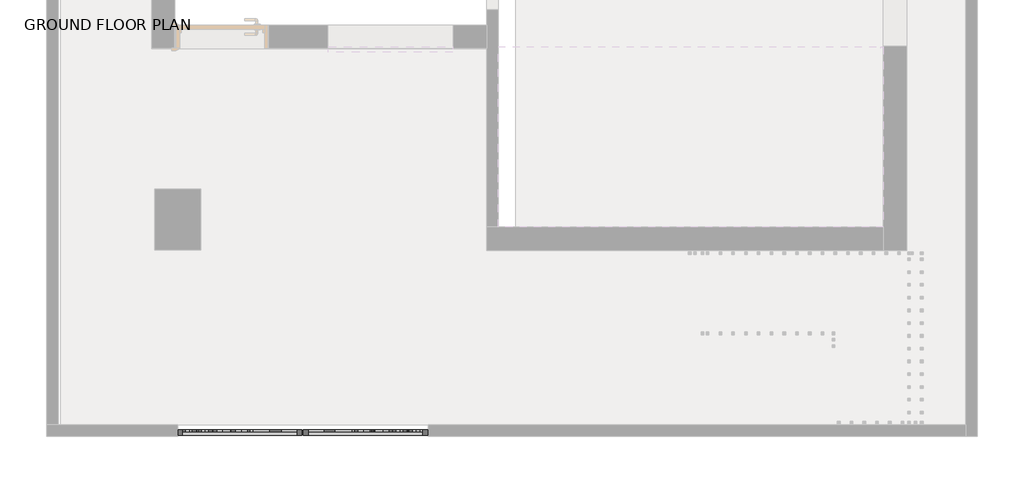
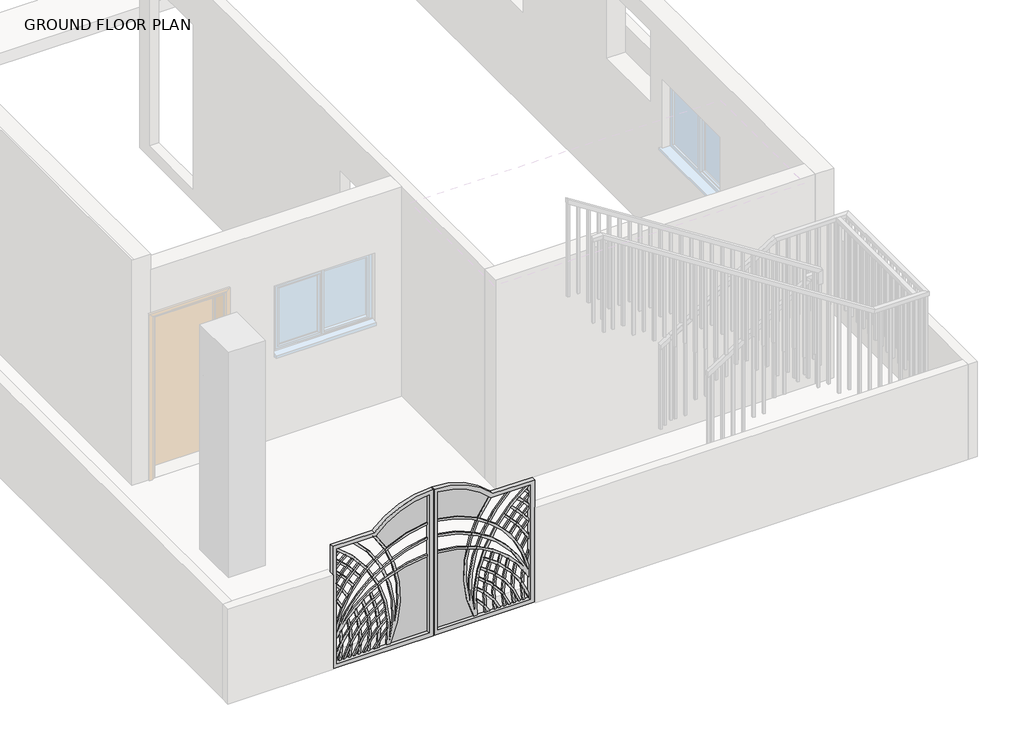
# One storey, part 23 of 23: 1 proxy, 1 railing.
"""IFC4 building model written with IfcOpenShell, lengths in millimetres."""

from ifc_helpers import new_model, si_unit, frame, origin, place, context, project, spatial, polyline, outline, extrude, faceted_brep, transform, mapped, element, save
from components import gate_7956_gate_7956_6bc30956

model = new_model("IFC4")

# Units and contexts
model_context = context("Model", 3, world=origin())
ifc_project = project(units=[si_unit("LENGTHUNIT", "METRE", prefix="MILLI")], contexts=[model_context])

# Site, building, storey
site = spatial("IfcSite", under=ifc_project)
building = spatial("IfcBuilding", under=site)
storey = spatial("IfcBuildingStorey", under=building, Name="GROUND FLOOR PLAN", Elevation=487.68)

# Proxy
placement = place(None, origin())
gate_7956_gate_7956_shape = gate_7956_gate_7956_6bc30956(model_context)
element("IfcBuildingElementProxy", 1, Name="gate_7956 : gate_7956", ObjectType="gate_7956 : gate_7956", at=placement, inside=storey, context=model_context, shape_type="MappedRepresentation", body=[
    mapped(gate_7956_gate_7956_shape, transform((-12591.4340108, -11978.9928911, 487.68), x_axis=(1.0, 0.0, 0.0), y_axis=(0.0, 1.0, 0.0), z_axis=(0.0, 0.0, 1.0))),
])

# Railing
element("IfcRailing", 2, ObjectType="1100mm", at=placement, inside=storey, context=model_context, shape_type="SolidModel", body=[
    faceted_brep([(-8805.870786, -10220.0521308, 1832.3649576), (-8805.870786, -10220.0521308, 1773.007357), (-8805.870786, -10270.0521308, 1773.007357), (-8805.870786, -10270.0521308, 1832.3649576), (-7409.7306254, -10220.0521308, 2725.6), (-7395.1045513, -10220.0521308, 2675.6), (-7395.1045513, -10270.0521308, 2675.6), (-7409.7306254, -10270.0521308, 2725.6), (-6621.5344696, -10220.0521308, 2725.6), (-6621.5344696, -10220.0521308, 2675.6), (-6671.5344696, -10270.0521308, 2675.6), (-6671.5344696, -10270.0521308, 2725.6), (-6621.5344696, -11933.6860066, 2725.6), (-6621.5344696, -11933.6860066, 2675.6), (-6671.5344696, -11883.6860066, 2675.6), (-6671.5344696, -11883.6860066, 2725.6), (-7155.718398, -11933.6860066, 2725.6), (-7170.3479429, -11933.6860066, 2675.6), (-7170.3479429, -11883.6860066, 2675.6), (-7155.718398, -11883.6860066, 2725.6), (-10457.8773536, -11933.6860066, 4838.88), (-10472.5068984, -11933.6860066, 4788.88), (-10472.5068984, -11883.6860066, 4788.88), (-10457.8773536, -11883.6860066, 4838.88), (-10583.5985666, -11933.6860066, 4838.88), (-10583.5985666, -11883.6860066, 4838.88), (-10583.5985666, -11883.6860066, 4788.88), (-10583.5985666, -11933.6860066, 4788.88)], [[[0, 1, 2, 3]], [[1, 0, 4, 5]], [[2, 1, 5, 6]], [[3, 2, 6, 7]], [[0, 3, 7, 4]], [[5, 4, 8, 9]], [[6, 5, 9, 10]], [[7, 6, 10, 11]], [[4, 7, 11, 8]], [[9, 8, 12, 13]], [[10, 9, 13, 14]], [[11, 10, 14, 15]], [[8, 11, 15, 12]], [[13, 12, 16, 17]], [[14, 13, 17, 18]], [[15, 14, 18, 19]], [[12, 15, 19, 16]], [[17, 16, 20, 21]], [[18, 17, 21, 22]], [[19, 18, 22, 23]], [[16, 19, 23, 20]], [[24, 25, 26, 27]], [[21, 20, 24, 27]], [[22, 21, 27, 26]], [[23, 22, 26, 25]], [[20, 23, 25, 24]]]),
    extrude(outline(polyline([(-10446.5344696, -11921.1860066), (-10471.5344696, -11921.1860066), (-10471.5344696, -11896.1860066), (-10446.5344696, -11896.1860066), (-10446.5344696, -11921.1860066)])), frame((0.0, 0.0, 3738.88), z_axis=(0.0, 0.0, 1.0), x_axis=(1.0, 0.0, 0.0)), (0.0, 0.0, 1.0), 1050.0),
    extrude(outline(polyline([(4692.2622966, -10321.5344696), (4708.2615264, -10346.5344696), (3576.32, -10346.5344696), (3576.32, -10321.5344696), (4692.2622966, -10321.5344696)])), frame((0.0, -11921.1860066, 0.0), z_axis=(0.0, 1.0, 0.0), x_axis=(0.0, 0.0, 1.0)), (0.0, 0.0, 1.0), 25.0),
    extrude(outline(polyline([(4612.2661476, -10196.5344696), (4628.2653774, -10221.5344696), (3576.32, -10221.5344696), (3576.32, -10196.5344696), (4612.2661476, -10196.5344696)])), frame((0.0, -11921.1860066, 0.0), z_axis=(0.0, 1.0, 0.0), x_axis=(0.0, 0.0, 1.0)), (0.0, 0.0, 1.0), 25.0),
    extrude(outline(polyline([(4532.2699985, -10071.5344696), (4548.2692283, -10096.5344696), (3413.76, -10096.5344696), (3413.76, -10071.5344696), (4532.2699985, -10071.5344696)])), frame((0.0, -11921.1860066, 0.0), z_axis=(0.0, 1.0, 0.0), x_axis=(0.0, 0.0, 1.0)), (0.0, 0.0, 1.0), 25.0),
    extrude(outline(polyline([(4452.2738495, -9946.5344696), (4468.2730793, -9971.5344696), (3413.76, -9971.5344696), (3413.76, -9946.5344696), (4452.2738495, -9946.5344696)])), frame((0.0, -11921.1860066, 0.0), z_axis=(0.0, 1.0, 0.0), x_axis=(0.0, 0.0, 1.0)), (0.0, 0.0, 1.0), 25.0),
    extrude(outline(polyline([(4372.2777004, -9821.5344696), (4388.2769302, -9846.5344696), (3251.2, -9846.5344696), (3251.2, -9821.5344696), (4372.2777004, -9821.5344696)])), frame((0.0, -11921.1860066, 0.0), z_axis=(0.0, 1.0, 0.0), x_axis=(0.0, 0.0, 1.0)), (0.0, 0.0, 1.0), 25.0),
    extrude(outline(polyline([(4292.2815514, -9696.5344696), (4308.2807812, -9721.5344696), (3251.2, -9721.5344696), (3251.2, -9696.5344696), (4292.2815514, -9696.5344696)])), frame((0.0, -11921.1860066, 0.0), z_axis=(0.0, 1.0, 0.0), x_axis=(0.0, 0.0, 1.0)), (0.0, 0.0, 1.0), 25.0),
    extrude(outline(polyline([(4212.2854023, -9571.5344696), (4228.2846321, -9596.5344696), (3088.64, -9596.5344696), (3088.64, -9571.5344696), (4212.2854023, -9571.5344696)])), frame((0.0, -11921.1860066, 0.0), z_axis=(0.0, 1.0, 0.0), x_axis=(0.0, 0.0, 1.0)), (0.0, 0.0, 1.0), 25.0),
    extrude(outline(polyline([(4132.2892533, -9446.5344696), (4148.2884831, -9471.5344696), (3088.64, -9471.5344696), (3088.64, -9446.5344696), (4132.2892533, -9446.5344696)])), frame((0.0, -11921.1860066, 0.0), z_axis=(0.0, 1.0, 0.0), x_axis=(0.0, 0.0, 1.0)), (0.0, 0.0, 1.0), 25.0),
    extrude(outline(polyline([(4052.2931042, -9321.5344696), (4068.292334, -9346.5344696), (2926.08, -9346.5344696), (2926.08, -9321.5344696), (4052.2931042, -9321.5344696)])), frame((0.0, -11921.1860066, 0.0), z_axis=(0.0, 1.0, 0.0), x_axis=(0.0, 0.0, 1.0)), (0.0, 0.0, 1.0), 25.0),
    extrude(outline(polyline([(3972.2969552, -9196.5344696), (3988.296185, -9221.5344696), (2926.08, -9221.5344696), (2926.08, -9196.5344696), (3972.2969552, -9196.5344696)])), frame((0.0, -11921.1860066, 0.0), z_axis=(0.0, 1.0, 0.0), x_axis=(0.0, 0.0, 1.0)), (0.0, 0.0, 1.0), 25.0),
    extrude(outline(polyline([(3892.3008061, -9071.5344696), (3908.3000359, -9096.5344696), (2763.52, -9096.5344696), (2763.52, -9071.5344696), (3892.3008061, -9071.5344696)])), frame((0.0, -11921.1860066, 0.0), z_axis=(0.0, 1.0, 0.0), x_axis=(0.0, 0.0, 1.0)), (0.0, 0.0, 1.0), 25.0),
    extrude(outline(polyline([(3812.3046571, -8946.5344696), (3828.3038869, -8971.5344696), (2763.52, -8971.5344696), (2763.52, -8946.5344696), (3812.3046571, -8946.5344696)])), frame((0.0, -11921.1860066, 0.0), z_axis=(0.0, 1.0, 0.0), x_axis=(0.0, 0.0, 1.0)), (0.0, 0.0, 1.0), 25.0),
    extrude(outline(polyline([(3732.308508, -8821.5344696), (3748.3077378, -8846.5344696), (2600.96, -8846.5344696), (2600.96, -8821.5344696), (3732.308508, -8821.5344696)])), frame((0.0, -11921.1860066, 0.0), z_axis=(0.0, 1.0, 0.0), x_axis=(0.0, 0.0, 1.0)), (0.0, 0.0, 1.0), 25.0),
    extrude(outline(polyline([(3652.312359, -8696.5344696), (3668.3115888, -8721.5344696), (2600.96, -8721.5344696), (2600.96, -8696.5344696), (3652.312359, -8696.5344696)])), frame((0.0, -11921.1860066, 0.0), z_axis=(0.0, 1.0, 0.0), x_axis=(0.0, 0.0, 1.0)), (0.0, 0.0, 1.0), 25.0),
    extrude(outline(polyline([(3572.3162099, -8571.5344696), (3588.3154397, -8596.5344696), (2438.4, -8596.5344696), (2438.4, -8571.5344696), (3572.3162099, -8571.5344696)])), frame((0.0, -11921.1860066, 0.0), z_axis=(0.0, 1.0, 0.0), x_axis=(0.0, 0.0, 1.0)), (0.0, 0.0, 1.0), 25.0),
    extrude(outline(polyline([(3492.3200609, -8446.5344696), (3508.3192907, -8471.5344696), (2438.4, -8471.5344696), (2438.4, -8446.5344696), (3492.3200609, -8446.5344696)])), frame((0.0, -11921.1860066, 0.0), z_axis=(0.0, 1.0, 0.0), x_axis=(0.0, 0.0, 1.0)), (0.0, 0.0, 1.0), 25.0),
    extrude(outline(polyline([(3412.3239118, -8321.5344696), (3428.3231416, -8346.5344696), (2275.84, -8346.5344696), (2275.84, -8321.5344696), (3412.3239118, -8321.5344696)])), frame((0.0, -11921.1860066, 0.0), z_axis=(0.0, 1.0, 0.0), x_axis=(0.0, 0.0, 1.0)), (0.0, 0.0, 1.0), 25.0),
    extrude(outline(polyline([(3332.3277628, -8196.5344696), (3348.3269926, -8221.5344696), (2275.84, -8221.5344696), (2275.84, -8196.5344696), (3332.3277628, -8196.5344696)])), frame((0.0, -11921.1860066, 0.0), z_axis=(0.0, 1.0, 0.0), x_axis=(0.0, 0.0, 1.0)), (0.0, 0.0, 1.0), 25.0),
    extrude(outline(polyline([(3252.3316137, -8071.5344696), (3268.3308435, -8096.5344696), (2113.28, -8096.5344696), (2113.28, -8071.5344696), (3252.3316137, -8071.5344696)])), frame((0.0, -11921.1860066, 0.0), z_axis=(0.0, 1.0, 0.0), x_axis=(0.0, 0.0, 1.0)), (0.0, 0.0, 1.0), 25.0),
    extrude(outline(polyline([(3172.3354647, -7946.5344696), (3188.3346945, -7971.5344696), (2113.28, -7971.5344696), (2113.28, -7946.5344696), (3172.3354647, -7946.5344696)])), frame((0.0, -11921.1860066, 0.0), z_axis=(0.0, 1.0, 0.0), x_axis=(0.0, 0.0, 1.0)), (0.0, 0.0, 1.0), 25.0),
    extrude(outline(polyline([(3092.4129874, -7821.5344696), (3108.4077111, -7846.5344696), (1950.72, -7846.5344696), (1950.72, -7821.5344696), (3092.4129874, -7821.5344696)])), frame((0.0, -11921.1860066, 0.0), z_axis=(0.0, 1.0, 0.0), x_axis=(0.0, 0.0, 1.0)), (0.0, 0.0, 1.0), 25.0),
    extrude(outline(polyline([(3012.4393691, -7696.5344696), (3028.4340928, -7721.5344696), (1950.72, -7721.5344696), (1950.72, -7696.5344696), (3012.4393691, -7696.5344696)])), frame((0.0, -11921.1860066, 0.0), z_axis=(0.0, 1.0, 0.0), x_axis=(0.0, 0.0, 1.0)), (0.0, 0.0, 1.0), 25.0),
    extrude(outline(polyline([(2932.4657508, -7571.5344696), (2948.4604745, -7596.5344696), (1788.16, -7596.5344696), (1788.16, -7571.5344696), (2932.4657508, -7571.5344696)])), frame((0.0, -11921.1860066, 0.0), z_axis=(0.0, 1.0, 0.0), x_axis=(0.0, 0.0, 1.0)), (0.0, 0.0, 1.0), 25.0),
    extrude(outline(polyline([(2852.4921325, -7446.5344696), (2868.4868562, -7471.5344696), (1788.16, -7471.5344696), (1788.16, -7446.5344696), (2852.4921325, -7446.5344696)])), frame((0.0, -11921.1860066, 0.0), z_axis=(0.0, 1.0, 0.0), x_axis=(0.0, 0.0, 1.0)), (0.0, 0.0, 1.0), 25.0),
    extrude(outline(polyline([(2772.3547194, -7321.5344696), (2788.3539492, -7346.5344696), (1625.6, -7346.5344696), (1625.6, -7321.5344696), (2772.3547194, -7321.5344696)])), frame((0.0, -11921.1860066, 0.0), z_axis=(0.0, 1.0, 0.0), x_axis=(0.0, 0.0, 1.0)), (0.0, 0.0, 1.0), 25.0),
    extrude(outline(polyline([(2692.3585703, -7196.5344696), (2708.3578001, -7221.5344696), (1625.6, -7221.5344696), (1625.6, -7196.5344696), (2692.3585703, -7196.5344696)])), frame((0.0, -11921.1860066, 0.0), z_axis=(0.0, 1.0, 0.0), x_axis=(0.0, 0.0, 1.0)), (0.0, 0.0, 1.0), 25.0),
    extrude(outline(polyline([(-7071.5344696, -11921.1860066), (-7096.5344696, -11921.1860066), (-7096.5344696, -11896.1860066), (-7071.5344696, -11896.1860066), (-7071.5344696, -11921.1860066)])), frame((0.0, 0.0, 1625.6), z_axis=(0.0, 0.0, 1.0), x_axis=(1.0, 0.0, 0.0)), (0.0, 0.0, 1.0), 1050.0),
    extrude(outline(polyline([(-6946.5344696, -11921.1860066), (-6971.5344696, -11921.1860066), (-6971.5344696, -11896.1860066), (-6946.5344696, -11896.1860066), (-6946.5344696, -11921.1860066)])), frame((0.0, 0.0, 1625.6), z_axis=(0.0, 0.0, 1.0), x_axis=(1.0, 0.0, 0.0)), (0.0, 0.0, 1.0), 1050.0),
    extrude(outline(polyline([(-6821.5344696, -11921.1860066), (-6846.5344696, -11921.1860066), (-6846.5344696, -11896.1860066), (-6821.5344696, -11896.1860066), (-6821.5344696, -11921.1860066)])), frame((0.0, 0.0, 1625.6), z_axis=(0.0, 0.0, 1.0), x_axis=(1.0, 0.0, 0.0)), (0.0, 0.0, 1.0), 1050.0),
    extrude(outline(polyline([(-6696.5344696, -11921.1860066), (-6721.5344696, -11921.1860066), (-6721.5344696, -11896.1860066), (-6696.5344696, -11896.1860066), (-6696.5344696, -11921.1860066)])), frame((0.0, 0.0, 1625.6), z_axis=(0.0, 0.0, 1.0), x_axis=(1.0, 0.0, 0.0)), (0.0, 0.0, 1.0), 1050.0),
    extrude(outline(polyline([(-6634.0344696, -11795.0521308), (-6634.0344696, -11820.0521308), (-6659.0344696, -11820.0521308), (-6659.0344696, -11795.0521308), (-6634.0344696, -11795.0521308)])), frame((0.0, 0.0, 1625.6), z_axis=(0.0, 0.0, 1.0), x_axis=(1.0, 0.0, 0.0)), (0.0, 0.0, 1.0), 1050.0),
    extrude(outline(polyline([(-6634.0344696, -11670.0521308), (-6634.0344696, -11695.0521308), (-6659.0344696, -11695.0521308), (-6659.0344696, -11670.0521308), (-6634.0344696, -11670.0521308)])), frame((0.0, 0.0, 1625.6), z_axis=(0.0, 0.0, 1.0), x_axis=(1.0, 0.0, 0.0)), (0.0, 0.0, 1.0), 1050.0),
    extrude(outline(polyline([(-6634.0344696, -11545.0521308), (-6634.0344696, -11570.0521308), (-6659.0344696, -11570.0521308), (-6659.0344696, -11545.0521308), (-6634.0344696, -11545.0521308)])), frame((0.0, 0.0, 1625.6), z_axis=(0.0, 0.0, 1.0), x_axis=(1.0, 0.0, 0.0)), (0.0, 0.0, 1.0), 1050.0),
    extrude(outline(polyline([(-6634.0344696, -11420.0521308), (-6634.0344696, -11445.0521308), (-6659.0344696, -11445.0521308), (-6659.0344696, -11420.0521308), (-6634.0344696, -11420.0521308)])), frame((0.0, 0.0, 1625.6), z_axis=(0.0, 0.0, 1.0), x_axis=(1.0, 0.0, 0.0)), (0.0, 0.0, 1.0), 1050.0),
    extrude(outline(polyline([(-6634.0344696, -11295.0521308), (-6634.0344696, -11320.0521308), (-6659.0344696, -11320.0521308), (-6659.0344696, -11295.0521308), (-6634.0344696, -11295.0521308)])), frame((0.0, 0.0, 1625.6), z_axis=(0.0, 0.0, 1.0), x_axis=(1.0, 0.0, 0.0)), (0.0, 0.0, 1.0), 1050.0),
    extrude(outline(polyline([(-6634.0344696, -11170.0521308), (-6634.0344696, -11195.0521308), (-6659.0344696, -11195.0521308), (-6659.0344696, -11170.0521308), (-6634.0344696, -11170.0521308)])), frame((0.0, 0.0, 1625.6), z_axis=(0.0, 0.0, 1.0), x_axis=(1.0, 0.0, 0.0)), (0.0, 0.0, 1.0), 1050.0),
    extrude(outline(polyline([(-6634.0344696, -11045.0521308), (-6634.0344696, -11070.0521308), (-6659.0344696, -11070.0521308), (-6659.0344696, -11045.0521308), (-6634.0344696, -11045.0521308)])), frame((0.0, 0.0, 1625.6), z_axis=(0.0, 0.0, 1.0), x_axis=(1.0, 0.0, 0.0)), (0.0, 0.0, 1.0), 1050.0),
    extrude(outline(polyline([(-6634.0344696, -10920.0521308), (-6634.0344696, -10945.0521308), (-6659.0344696, -10945.0521308), (-6659.0344696, -10920.0521308), (-6634.0344696, -10920.0521308)])), frame((0.0, 0.0, 1625.6), z_axis=(0.0, 0.0, 1.0), x_axis=(1.0, 0.0, 0.0)), (0.0, 0.0, 1.0), 1050.0),
    extrude(outline(polyline([(-6634.0344696, -10795.0521308), (-6634.0344696, -10820.0521308), (-6659.0344696, -10820.0521308), (-6659.0344696, -10795.0521308), (-6634.0344696, -10795.0521308)])), frame((0.0, 0.0, 1625.6), z_axis=(0.0, 0.0, 1.0), x_axis=(1.0, 0.0, 0.0)), (0.0, 0.0, 1.0), 1050.0),
    extrude(outline(polyline([(-6634.0344696, -10670.0521308), (-6634.0344696, -10695.0521308), (-6659.0344696, -10695.0521308), (-6659.0344696, -10670.0521308), (-6634.0344696, -10670.0521308)])), frame((0.0, 0.0, 1625.6), z_axis=(0.0, 0.0, 1.0), x_axis=(1.0, 0.0, 0.0)), (0.0, 0.0, 1.0), 1050.0),
    extrude(outline(polyline([(-6634.0344696, -10545.0521308), (-6634.0344696, -10570.0521308), (-6659.0344696, -10570.0521308), (-6659.0344696, -10545.0521308), (-6634.0344696, -10545.0521308)])), frame((0.0, 0.0, 1625.6), z_axis=(0.0, 0.0, 1.0), x_axis=(1.0, 0.0, 0.0)), (0.0, 0.0, 1.0), 1050.0),
    extrude(outline(polyline([(-6634.0344696, -10420.0521308), (-6634.0344696, -10445.0521308), (-6659.0344696, -10445.0521308), (-6659.0344696, -10420.0521308), (-6634.0344696, -10420.0521308)])), frame((0.0, 0.0, 1625.6), z_axis=(0.0, 0.0, 1.0), x_axis=(1.0, 0.0, 0.0)), (0.0, 0.0, 1.0), 1050.0),
    extrude(outline(polyline([(-6634.0344696, -10295.0521308), (-6634.0344696, -10320.0521308), (-6659.0344696, -10320.0521308), (-6659.0344696, -10295.0521308), (-6634.0344696, -10295.0521308)])), frame((0.0, 0.0, 1625.6), z_axis=(0.0, 0.0, 1.0), x_axis=(1.0, 0.0, 0.0)), (0.0, 0.0, 1.0), 1050.0),
    extrude(outline(polyline([(-6755.870786, -10232.5521308), (-6730.870786, -10232.5521308), (-6730.870786, -10257.5521308), (-6755.870786, -10257.5521308), (-6755.870786, -10232.5521308)])), frame((0.0, 0.0, 1625.6), z_axis=(0.0, 0.0, 1.0), x_axis=(1.0, 0.0, 0.0)), (0.0, 0.0, 1.0), 1050.0),
    extrude(outline(polyline([(-6880.870786, -10232.5521308), (-6855.870786, -10232.5521308), (-6855.870786, -10257.5521308), (-6880.870786, -10257.5521308), (-6880.870786, -10232.5521308)])), frame((0.0, 0.0, 1625.6), z_axis=(0.0, 0.0, 1.0), x_axis=(1.0, 0.0, 0.0)), (0.0, 0.0, 1.0), 1050.0),
    extrude(outline(polyline([(-7005.870786, -10232.5521308), (-6980.870786, -10232.5521308), (-6980.870786, -10257.5521308), (-7005.870786, -10257.5521308), (-7005.870786, -10232.5521308)])), frame((0.0, 0.0, 1625.6), z_axis=(0.0, 0.0, 1.0), x_axis=(1.0, 0.0, 0.0)), (0.0, 0.0, 1.0), 1050.0),
    extrude(outline(polyline([(-7130.870786, -10232.5521308), (-7105.870786, -10232.5521308), (-7105.870786, -10257.5521308), (-7130.870786, -10257.5521308), (-7130.870786, -10232.5521308)])), frame((0.0, 0.0, 1625.6), z_axis=(0.0, 0.0, 1.0), x_axis=(1.0, 0.0, 0.0)), (0.0, 0.0, 1.0), 1050.0),
    extrude(outline(polyline([(-7255.870786, -10232.5521308), (-7230.870786, -10232.5521308), (-7230.870786, -10257.5521308), (-7255.870786, -10257.5521308), (-7255.870786, -10232.5521308)])), frame((0.0, 0.0, 1625.6), z_axis=(0.0, 0.0, 1.0), x_axis=(1.0, 0.0, 0.0)), (0.0, 0.0, 1.0), 1050.0),
    extrude(outline(polyline([(-7380.870786, -10232.5521308), (-7355.870786, -10232.5521308), (-7355.870786, -10257.5521308), (-7380.870786, -10257.5521308), (-7380.870786, -10232.5521308)])), frame((0.0, 0.0, 1625.6), z_axis=(0.0, 0.0, 1.0), x_axis=(1.0, 0.0, 0.0)), (0.0, 0.0, 1.0), 1050.0),
    extrude(outline(polyline([(1463.04, -7505.870786), (1463.04, -7480.870786), (2620.7277111, -7480.870786), (2604.7329874, -7505.870786), (1463.04, -7505.870786)])), frame((0.0, -10257.5521308, 0.0), z_axis=(0.0, 1.0, 0.0), x_axis=(0.0, 0.0, 1.0)), (0.0, 0.0, 1.0), 25.0),
    extrude(outline(polyline([(1463.04, -7630.870786), (1463.04, -7605.870786), (2540.7540928, -7605.870786), (2524.7593691, -7630.870786), (1463.04, -7630.870786)])), frame((0.0, -10257.5521308, 0.0), z_axis=(0.0, 1.0, 0.0), x_axis=(0.0, 0.0, 1.0)), (0.0, 0.0, 1.0), 25.0),
    extrude(outline(polyline([(1300.48, -7755.870786), (1300.48, -7730.870786), (2460.7804745, -7730.870786), (2444.7857508, -7755.870786), (1300.48, -7755.870786)])), frame((0.0, -10257.5521308, 0.0), z_axis=(0.0, 1.0, 0.0), x_axis=(0.0, 0.0, 1.0)), (0.0, 0.0, 1.0), 25.0),
    extrude(outline(polyline([(1300.48, -7880.870786), (1300.48, -7855.870786), (2380.8068562, -7855.870786), (2364.8121325, -7880.870786), (1300.48, -7880.870786)])), frame((0.0, -10257.5521308, 0.0), z_axis=(0.0, 1.0, 0.0), x_axis=(0.0, 0.0, 1.0)), (0.0, 0.0, 1.0), 25.0),
    extrude(outline(polyline([(1137.92, -8005.870786), (1137.92, -7980.870786), (2300.8332379, -7980.870786), (2284.8385142, -8005.870786), (1137.92, -8005.870786)])), frame((0.0, -10257.5521308, 0.0), z_axis=(0.0, 1.0, 0.0), x_axis=(0.0, 0.0, 1.0)), (0.0, 0.0, 1.0), 25.0),
    extrude(outline(polyline([(1137.92, -8130.870786), (1137.92, -8105.870786), (2220.8596196, -8105.870786), (2204.8648959, -8130.870786), (1137.92, -8130.870786)])), frame((0.0, -10257.5521308, 0.0), z_axis=(0.0, 1.0, 0.0), x_axis=(0.0, 0.0, 1.0)), (0.0, 0.0, 1.0), 25.0),
    extrude(outline(polyline([(975.36, -8255.870786), (975.36, -8230.870786), (2140.8860012, -8230.870786), (2124.8912776, -8255.870786), (975.36, -8255.870786)])), frame((0.0, -10257.5521308, 0.0), z_axis=(0.0, 1.0, 0.0), x_axis=(0.0, 0.0, 1.0)), (0.0, 0.0, 1.0), 25.0),
    extrude(outline(polyline([(975.36, -8380.870786), (975.36, -8355.870786), (2060.9123829, -8355.870786), (2044.9176593, -8380.870786), (975.36, -8380.870786)])), frame((0.0, -10257.5521308, 0.0), z_axis=(0.0, 1.0, 0.0), x_axis=(0.0, 0.0, 1.0)), (0.0, 0.0, 1.0), 25.0),
    extrude(outline(polyline([(812.8, -8505.870786), (812.8, -8480.870786), (1980.9387646, -8480.870786), (1964.944041, -8505.870786), (812.8, -8505.870786)])), frame((0.0, -10257.5521308, 0.0), z_axis=(0.0, 1.0, 0.0), x_axis=(0.0, 0.0, 1.0)), (0.0, 0.0, 1.0), 25.0),
    extrude(outline(polyline([(812.8, -8630.870786), (812.8, -8605.870786), (1900.9651463, -8605.870786), (1884.9704227, -8630.870786), (812.8, -8630.870786)])), frame((0.0, -10257.5521308, 0.0), z_axis=(0.0, 1.0, 0.0), x_axis=(0.0, 0.0, 1.0)), (0.0, 0.0, 1.0), 25.0),
    extrude(outline(polyline([(772.3517667, -8755.870786), (772.3517667, -8730.870786), (1820.991528, -8730.870786), (1804.9968044, -8755.870786), (772.3517667, -8755.870786)])), frame((0.0, -10257.5521308, 0.0), z_axis=(0.0, 1.0, 0.0), x_axis=(0.0, 0.0, 1.0)), (0.0, 0.0, 1.0), 25.0),
    extrude(outline(polyline([(-6634.0344696, -11896.1860066), (-6634.0344696, -11921.1860066), (-6659.0344696, -11921.1860066), (-6659.0344696, -11896.1860066), (-6634.0344696, -11896.1860066)])), frame((0.0, 0.0, 1625.6), z_axis=(0.0, 0.0, 1.0), x_axis=(1.0, 0.0, 0.0)), (0.0, 0.0, 1.0), 1050.0),
    extrude(outline(polyline([(-6659.0344696, -10232.5521308), (-6634.0344696, -10232.5521308), (-6634.0344696, -10257.5521308), (-6659.0344696, -10257.5521308), (-6659.0344696, -10232.5521308)])), frame((0.0, 0.0, 1625.6), z_axis=(0.0, 0.0, 1.0), x_axis=(1.0, 0.0, 0.0)), (0.0, 0.0, 1.0), 1050.0),
    extrude(outline(polyline([(-10558.5985666, -11921.1860066), (-10583.5985666, -11921.1860066), (-10583.5985666, -11896.1860066), (-10558.5985666, -11896.1860066), (-10558.5985666, -11921.1860066)])), frame((0.0, 0.0, 3738.88), z_axis=(0.0, 0.0, 1.0), x_axis=(1.0, 0.0, 0.0)), (0.0, 0.0, 1.0), 1050.0),
    extrude(outline(polyline([(740.3623194, -8805.870786), (740.3623194, -8780.870786), (1789.0020807, -8780.870786), (1773.007357, -8805.870786), (740.3623194, -8805.870786)])), frame((0.0, -10257.5521308, 0.0), z_axis=(0.0, 1.0, 0.0), x_axis=(0.0, 0.0, 1.0)), (0.0, 0.0, 1.0), 25.0),
])

save(model, "model.ifc")

# Revit data of these elements
# Type "gate_7956 : gate_7956"
#   m.s. sheet = none
#   2" x2" pipe = none
#   1"x1"pipe = none
#   Default Elevation = 0
# Type "1100mm"
#   built-in parameter 1008612 = 0.019685 (stored number, unit not read)
#   built-in parameter 1008611 = 0.019685 (stored number, unit not read)
#   built-in parameter 1008609 = 0.902231 (stored number, unit not read)
#   built-in parameter 1008604 = 0.19685 (stored number, unit not read)
#   built-in parameter 1008603 = 0.164042 (stored number, unit not read)
#   Railing Height = 3.608924 ft
#   built-in parameter 1008630 = 2
#   built-in parameter 1008610 = 2
#   built-in parameter 1008608 = 1
#   built-in parameter 1008618 = Baluster_Square : 25mm
# Element 1 (IfcBuildingElementProxy, "gate_7956 : gate_7956")
#   Phase Created = New Construction
# Element 2 (IfcRailing, "1100mm")
#   Phase Created = New Construction
